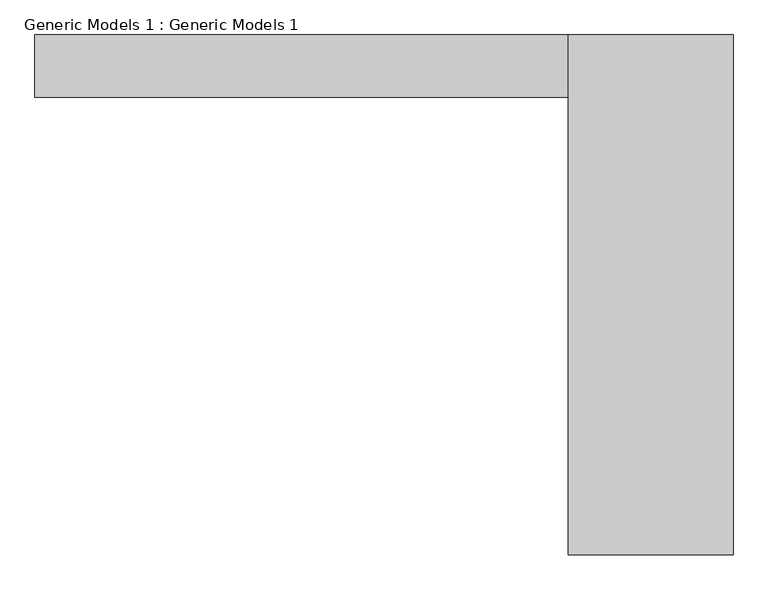
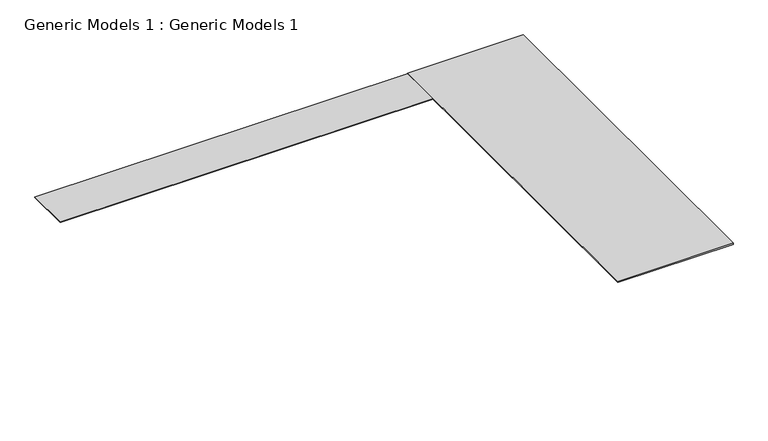
"""IFC4 building model written with IfcOpenShell, lengths in millimetres: proxy geometry, Generic Models 1 : Generic Models 1."""

from ifc_helpers import new_model, si_unit, frame, origin, place, context, project, spatial, polyline, outline, extrude, source, transform, mapped, element, save


def generic_models_1_generic_models_1_c6e5ea94(model_context):
    return source(origin(), model_context, "Body", "SweptSolid", [
        extrude(outline(polyline([(16465.7514396, 14964.4892668), (-13557.0485604, 14964.4892668), (-13557.0485604, 18469.6892668), (16465.7514396, 18469.6892668), (16465.7514396, 14964.4892668)])), frame((0.0, 0.0, -76.2), z_axis=(0.0, 0.0, 1.0), x_axis=(1.0, 0.0, 0.0)), (0.0, 0.0, 1.0), 26.6960077),
        extrude(outline(polyline([(25752.720019, 18469.6892668), (25752.720019, -10791.1107332), (16465.7514396, -10791.1107332), (16465.7514396, 18469.6892668), (25752.720019, 18469.6892668)])), frame((0.0, 0.0, -76.2), z_axis=(0.0, 0.0, 1.0), x_axis=(1.0, 0.0, 0.0)), (0.0, 0.0, 1.0), 94.2951867),
    ])


if __name__ == "__main__":
    model = new_model("IFC4")
    model_context = context("Model", 3, world=origin())
    ifc_project = project(units=[si_unit("LENGTHUNIT", "METRE", prefix="MILLI")], contexts=[model_context])
    site = spatial("IfcSite", under=ifc_project)
    building = spatial("IfcBuilding", under=site)
    placement = place(None, origin())
    generic_models_1_generic_models_1_shape = generic_models_1_generic_models_1_c6e5ea94(model_context)
    element("IfcBuildingElementProxy", 1, Name="Generic Models 1 : Generic Models 1", ObjectType="Generic Models 1 : Generic Models 1", at=placement, inside=building, context=model_context, shape_type="MappedRepresentation", body=[
        mapped(generic_models_1_generic_models_1_shape, transform((0.0, 0.0, 0.0), x_axis=(1.0, 0.0, 0.0), y_axis=(0.0, 1.0, 0.0), z_axis=(0.0, 0.0, 1.0))),
    ])
    save(model, "model.ifc")
